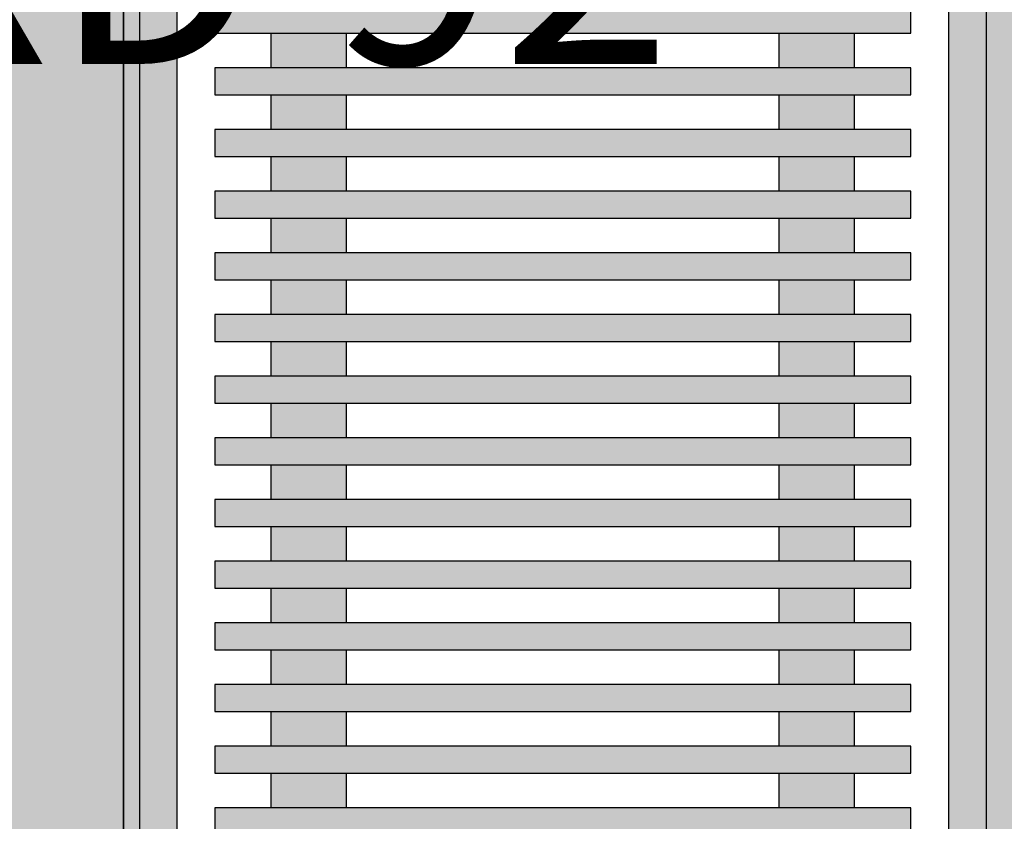
# Model space of a CAD drawing. Units: inches. Extents: x 1704 to 6393, y -157 to 1172.
# Tile 28 of 122: x 2351 to 2377, y 295 to 316. Entities that reach past the tile are written whole.
import ezdxf

# ---------------------------------------------------------------- set-up
doc = ezdxf.new("R2010")
doc.units = ezdxf.units.IN
doc.header["$MEASUREMENT"] = 0
for name, color, linetype, lineweight in [('A-ANNO-DIMS', 7, 'Continuous', 13), ('A-FURN', 8, 'Continuous', 18), ('A-WALL-PATT', 7, 'Continuous', 13), ('estofado', 7, 'Continuous', 25), ('WALLS', 7, 'Continuous', 35)]:
    doc.layers.add(name, color=color, linetype=linetype, lineweight=lineweight)
doc.layers.add('A-FLOR-PATT', color=7, linetype='Continuous', lineweight=13, true_color=0xf2f2f2)
doc.layers.add('MOBIL', color=7, linetype='Continuous')
doc.styles.get("Standard").update_dxf_attribs({"font": 'arial.ttf'})
doc.dimstyles.get("Standard").update_dxf_attribs({"dimtxt": 6, "dimasz": 2, "dimexe": 0.18, "dimexo": 0.0625, "dimgap": 0.09, "dimtad": 0, "dimtih": 1, "dimtoh": 1, "dimdec": 1, "dimzin": 0, "dimdsep": 46, "dimlunit": 3, "dimtxsty": 'Standard', "dimblk": 'ARCHTICK', "dimcen": 0.09, "dimadec": 0, "dimazin": 0, "dimtfac": 1, "dimtdec": 1, "dimtofl": 0, "dimtmove": 0, "dimatfit": 3, "dimfxl": 1, "dimtolj": 1, "dimtzin": 0, "dimarcsym": 0})

# ---------------------------------------------------------------- blocks, each defined once
blk = doc.blocks.new('Aparador Aido WV')
at = {"layer": 'MOBIL'}
h = blk.add_hatch(color=256, dxfattribs=at)
h.set_gradient(color1=(226, 228, 228), one_color=1, tint=1, name='CYLINDER')
h.paths.add_polyline_path([(0.9, -0.02), (0.9, 0), (-0.9, 0), (-0.9, -0.02)])
h = blk.add_hatch(color=256, dxfattribs=at)
h.set_gradient(color1=(106, 79, 62), color2=(55, 41, 32), one_color=1, tint=0.17)
h.paths.add_polyline_path([(-0.4692, -0.04017), (-0.4692, -0.40983), (-0.45483, -0.40983), (-0.45483, -0.04017)])
h = blk.add_hatch(color=256, dxfattribs=at)
h.set_gradient(color1=(106, 79, 62), color2=(55, 41, 32), one_color=1, tint=0.17)
h.paths.add_polyline_path([(-0.43644, -0.04017), (-0.43644, -0.40983), (-0.42208, -0.40983), (-0.42208, -0.04017)])
h = blk.add_hatch(color=256, dxfattribs=at)
h.set_gradient(color1=(106, 79, 62), color2=(55, 41, 32), one_color=1, tint=0.17)
h.paths.add_polyline_path([(-0.40369, -0.04017), (-0.40369, -0.40983), (-0.38933, -0.40983), (-0.38933, -0.04017)])
h = blk.add_hatch(color=256, dxfattribs=at)
h.set_gradient(color1=(106, 79, 62), color2=(55, 41, 32), one_color=1, tint=0.17)
h.paths.add_polyline_path([(-0.37094, -0.04017), (-0.37094, -0.40983), (-0.35658, -0.40983), (-0.35658, -0.04017)])
h = blk.add_hatch(color=256, dxfattribs=at)
h.set_gradient(color1=(106, 79, 62), color2=(55, 41, 32), one_color=1, tint=0.17)
h.paths.add_polyline_path([(-0.33819, -0.04017), (-0.33819, -0.40983), (-0.32382, -0.40983), (-0.32382, -0.04017)])
h = blk.add_hatch(color=256, dxfattribs=at)
h.set_gradient(color1=(106, 79, 62), color2=(55, 41, 32), one_color=1, tint=0.17)
h.paths.add_polyline_path([(-0.30544, -0.04017), (-0.30544, -0.40983), (-0.29107, -0.40983), (-0.29107, -0.04017)])
h = blk.add_hatch(color=256, dxfattribs=at)
h.set_gradient(color1=(106, 79, 62), color2=(55, 41, 32), one_color=1, tint=0.17)
h.paths.add_polyline_path([(-0.27269, -0.04017), (-0.27269, -0.40983), (-0.25832, -0.40983), (-0.25832, -0.04017)])
h = blk.add_hatch(color=256, dxfattribs=at)
h.set_gradient(color1=(106, 79, 62), color2=(55, 41, 32), one_color=1, tint=0.17)
h.paths.add_polyline_path([(-0.23993, -0.04017), (-0.23993, -0.40983), (-0.22557, -0.40983), (-0.22557, -0.04017)])
h = blk.add_hatch(color=256, dxfattribs=at)
h.set_gradient(color1=(106, 79, 62), color2=(55, 41, 32), one_color=1, tint=0.17)
h.paths.add_polyline_path([(-0.20718, -0.40983), (-0.19282, -0.40983), (-0.19282, -0.04017), (-0.20718, -0.04017)])
h = blk.add_hatch(color=256, dxfattribs=at)
h.set_gradient(color1=(106, 79, 62), color2=(55, 41, 32), one_color=1, tint=0.17)
h.paths.add_polyline_path([(-0.17443, -0.04017), (-0.17443, -0.40983), (-0.16007, -0.40983), (-0.16007, -0.04017)])
h = blk.add_hatch(color=256, dxfattribs=at)
h.set_gradient(color1=(106, 79, 62), color2=(55, 41, 32), one_color=1, tint=0.17)
h.paths.add_polyline_path([(-0.14168, -0.04017), (-0.14168, -0.40983), (-0.12731, -0.40983), (-0.12731, -0.04017)])
h = blk.add_hatch(color=256, dxfattribs=at)
h.set_gradient(color1=(106, 79, 62), color2=(55, 41, 32), one_color=1, tint=0.17)
h.paths.add_polyline_path([(-0.10893, -0.04017), (-0.10893, -0.40983), (-0.09456, -0.40983), (-0.09456, -0.04017)])
h = blk.add_hatch(color=256, dxfattribs=at)
h.set_gradient(color1=(106, 79, 62), color2=(55, 41, 32), one_color=1, tint=0.17)
h.paths.add_polyline_path([(-0.07618, -0.04017), (-0.07618, -0.40983), (-0.06181, -0.40983), (-0.06181, -0.04017)])
h = blk.add_hatch(color=256, dxfattribs=at)
h.set_gradient(color1=(106, 79, 62), color2=(55, 41, 32), one_color=1, tint=0.17)
h.paths.add_polyline_path([(-0.04342, -0.04017), (-0.04342, -0.40983), (-0.02906, -0.40983), (-0.02906, -0.04017)])
h = blk.add_hatch(color=256, dxfattribs=at)
h.set_gradient(color1=(106, 79, 62), color2=(157, 117, 92), one_color=1, tint=0.49)
h.paths.add_polyline_path([(-0.43644, -0.07), (-0.45483, -0.07), (-0.45483, -0.11), (-0.43644, -0.11)])
h = blk.add_hatch(color=256, dxfattribs=at)
h.set_gradient(color1=(106, 79, 62), color2=(157, 117, 92), one_color=1, tint=0.49)
h.paths.add_polyline_path([(-0.40369, -0.07), (-0.42208, -0.07), (-0.42208, -0.11), (-0.40369, -0.11)])
h = blk.add_hatch(color=256, dxfattribs=at)
h.set_gradient(color1=(106, 79, 62), color2=(157, 117, 92), one_color=1, tint=0.49)
h.paths.add_polyline_path([(-0.37094, -0.07), (-0.38933, -0.07), (-0.38933, -0.11), (-0.37094, -0.11)])
h = blk.add_hatch(color=256, dxfattribs=at)
h.set_gradient(color1=(106, 79, 62), color2=(157, 117, 92), one_color=1, tint=0.49)
h.paths.add_polyline_path([(-0.33819, -0.07), (-0.35658, -0.07), (-0.35658, -0.11), (-0.33819, -0.11)])
h = blk.add_hatch(color=256, dxfattribs=at)
h.set_gradient(color1=(106, 79, 62), color2=(157, 117, 92), one_color=1, tint=0.49)
h.paths.add_polyline_path([(-0.30544, -0.07), (-0.32382, -0.07), (-0.32382, -0.11), (-0.30544, -0.11)])
h = blk.add_hatch(color=256, dxfattribs=at)
h.set_gradient(color1=(106, 79, 62), color2=(157, 117, 92), one_color=1, tint=0.49)
h.paths.add_polyline_path([(-0.27269, -0.07), (-0.29107, -0.07), (-0.29107, -0.11), (-0.27269, -0.11)])
h = blk.add_hatch(color=256, dxfattribs=at)
h.set_gradient(color1=(106, 79, 62), color2=(157, 117, 92), one_color=1, tint=0.49)
h.paths.add_polyline_path([(-0.23993, -0.07), (-0.25832, -0.07), (-0.25832, -0.11), (-0.23993, -0.11)])
h = blk.add_hatch(color=256, dxfattribs=at)
h.set_gradient(color1=(106, 79, 62), color2=(157, 117, 92), one_color=1, tint=0.49)
h.paths.add_polyline_path([(-0.20718, -0.07), (-0.22557, -0.07), (-0.22557, -0.11), (-0.20718, -0.11)])
h = blk.add_hatch(color=256, dxfattribs=at)
h.set_gradient(color1=(106, 79, 62), color2=(157, 117, 92), one_color=1, tint=0.49)
h.paths.add_polyline_path([(-0.17443, -0.07), (-0.19282, -0.07), (-0.19282, -0.11), (-0.17443, -0.11)])
h = blk.add_hatch(color=256, dxfattribs=at)
h.set_gradient(color1=(106, 79, 62), color2=(157, 117, 92), one_color=1, tint=0.49)
h.paths.add_polyline_path([(-0.14168, -0.07), (-0.16007, -0.07), (-0.16007, -0.11), (-0.14168, -0.11)])
h = blk.add_hatch(color=256, dxfattribs=at)
h.set_gradient(color1=(106, 79, 62), color2=(157, 117, 92), one_color=1, tint=0.49)
h.paths.add_polyline_path([(-0.10893, -0.07), (-0.12731, -0.07), (-0.12731, -0.11), (-0.10893, -0.11)])
h = blk.add_hatch(color=256, dxfattribs=at)
h.set_gradient(color1=(106, 79, 62), color2=(157, 117, 92), one_color=1, tint=0.49)
h.paths.add_polyline_path([(-0.07618, -0.07), (-0.09456, -0.07), (-0.09456, -0.11), (-0.07618, -0.11)])
h = blk.add_hatch(color=256, dxfattribs=at)
h.set_gradient(color1=(106, 79, 62), color2=(157, 117, 92), one_color=1, tint=0.49)
h.paths.add_polyline_path([(-0.04342, -0.07), (-0.06181, -0.07), (-0.06181, -0.11), (-0.04342, -0.11)])
h = blk.add_hatch(color=256, dxfattribs=at)
h.set_gradient(color1=(106, 79, 62), color2=(157, 117, 92), one_color=1, tint=0.49)
h.paths.add_polyline_path([(-0.43644, -0.34), (-0.45483, -0.34), (-0.45483, -0.38), (-0.43644, -0.38)])
h = blk.add_hatch(color=256, dxfattribs=at)
h.set_gradient(color1=(106, 79, 62), color2=(157, 117, 92), one_color=1, tint=0.49)
h.paths.add_polyline_path([(-0.40369, -0.34), (-0.42208, -0.34), (-0.42208, -0.38), (-0.40369, -0.38)])
h = blk.add_hatch(color=256, dxfattribs=at)
h.set_gradient(color1=(106, 79, 62), color2=(157, 117, 92), one_color=1, tint=0.49)
h.paths.add_polyline_path([(-0.37094, -0.34), (-0.38933, -0.34), (-0.38933, -0.38), (-0.37094, -0.38)])
h = blk.add_hatch(color=256, dxfattribs=at)
h.set_gradient(color1=(106, 79, 62), color2=(157, 117, 92), one_color=1, tint=0.49)
h.paths.add_polyline_path([(-0.33819, -0.34), (-0.35658, -0.34), (-0.35658, -0.38), (-0.33819, -0.38)])
h = blk.add_hatch(color=256, dxfattribs=at)
h.set_gradient(color1=(106, 79, 62), color2=(157, 117, 92), one_color=1, tint=0.49)
h.paths.add_polyline_path([(-0.30544, -0.34), (-0.32382, -0.34), (-0.32382, -0.38), (-0.30544, -0.38)])
h = blk.add_hatch(color=256, dxfattribs=at)
h.set_gradient(color1=(106, 79, 62), color2=(157, 117, 92), one_color=1, tint=0.49)
h.paths.add_polyline_path([(-0.27269, -0.34), (-0.29107, -0.34), (-0.29107, -0.38), (-0.27269, -0.38)])
h = blk.add_hatch(color=256, dxfattribs=at)
h.set_gradient(color1=(106, 79, 62), color2=(157, 117, 92), one_color=1, tint=0.49)
h.paths.add_polyline_path([(-0.23993, -0.34), (-0.25832, -0.34), (-0.25832, -0.38), (-0.23993, -0.38)])
h = blk.add_hatch(color=256, dxfattribs=at)
h.set_gradient(color1=(106, 79, 62), color2=(157, 117, 92), one_color=1, tint=0.49)
h.paths.add_polyline_path([(-0.20718, -0.34), (-0.22557, -0.34), (-0.22557, -0.38), (-0.20718, -0.38)])
h = blk.add_hatch(color=256, dxfattribs=at)
h.set_gradient(color1=(106, 79, 62), color2=(157, 117, 92), one_color=1, tint=0.49)
h.paths.add_polyline_path([(-0.17443, -0.34), (-0.19282, -0.34), (-0.19282, -0.38), (-0.17443, -0.38)])
h = blk.add_hatch(color=256, dxfattribs=at)
h.set_gradient(color1=(106, 79, 62), color2=(157, 117, 92), one_color=1, tint=0.49)
h.paths.add_polyline_path([(-0.14168, -0.34), (-0.16007, -0.34), (-0.16007, -0.38), (-0.14168, -0.38)])
h = blk.add_hatch(color=256, dxfattribs=at)
h.set_gradient(color1=(106, 79, 62), color2=(157, 117, 92), one_color=1, tint=0.49)
h.paths.add_polyline_path([(-0.10893, -0.34), (-0.12731, -0.34), (-0.12731, -0.38), (-0.10893, -0.38)])
h = blk.add_hatch(color=256, dxfattribs=at)
h.set_gradient(color1=(106, 79, 62), color2=(157, 117, 92), one_color=1, tint=0.49)
h.paths.add_polyline_path([(-0.07618, -0.34), (-0.09456, -0.34), (-0.09456, -0.38), (-0.07618, -0.38)])
h = blk.add_hatch(color=256, dxfattribs=at)
h.set_gradient(color1=(106, 79, 62), color2=(157, 117, 92), one_color=1, tint=0.49)
h.paths.add_polyline_path([(-0.04342, -0.34), (-0.06181, -0.34), (-0.06181, -0.38), (-0.04342, -0.38)])
h = blk.add_hatch(color=256, dxfattribs=at)
h.set_gradient(color1=(226, 228, 228), one_color=1, tint=1, name='CYLINDER')
h.paths.add_polyline_path([(0.9, -0.45), (0.9, -0.43), (-0.9, -0.43), (-0.9, -0.45)])
at = {"layer": 'estofado', "ltscale": 0.5}
for p, q in [((-0.45483, -0.07), (-0.43644, -0.07)), ((-0.42208, -0.07), (-0.40369, -0.07)), ((-0.38933, -0.07), (-0.37094, -0.07)), ((-0.35658, -0.07), (-0.33819, -0.07)), ((-0.32382, -0.07), (-0.30544, -0.07)), ((-0.29107, -0.07), (-0.27269, -0.07)), ((-0.25832, -0.07), (-0.23993, -0.07)), ((-0.22557, -0.07), (-0.20718, -0.07)), ((-0.19282, -0.07), (-0.17443, -0.07)), ((-0.16007, -0.07), (-0.14168, -0.07)), ((-0.12731, -0.07), (-0.10893, -0.07)), ((-0.09456, -0.07), (-0.07618, -0.07)), ((-0.06181, -0.07), (-0.04342, -0.07)), ((-0.45483, -0.11), (-0.43644, -0.11)), ((-0.42208, -0.11), (-0.40369, -0.11)), ((-0.38933, -0.11), (-0.37094, -0.11)), ((-0.35658, -0.11), (-0.33819, -0.11)), ((-0.32382, -0.11), (-0.30544, -0.11)), ((-0.29107, -0.11), (-0.27269, -0.11)), ((-0.25832, -0.11), (-0.23993, -0.11)), ((-0.22557, -0.11), (-0.20718, -0.11)), ((-0.19282, -0.11), (-0.17443, -0.11)), ((-0.16007, -0.11), (-0.14168, -0.11)), ((-0.12731, -0.11), (-0.10893, -0.11)), ((-0.09456, -0.11), (-0.07618, -0.11)), ((-0.06181, -0.11), (-0.04342, -0.11)), ((-0.45483, -0.34), (-0.43644, -0.34)), ((-0.42208, -0.34), (-0.40369, -0.34)), ((-0.38933, -0.34), (-0.37094, -0.34)), ((-0.35658, -0.34), (-0.33819, -0.34)), ((-0.32382, -0.34), (-0.30544, -0.34)), ((-0.29107, -0.34), (-0.27269, -0.34)), ((-0.25832, -0.34), (-0.23993, -0.34)), ((-0.22557, -0.34), (-0.20718, -0.34)), ((-0.19282, -0.34), (-0.17443, -0.34)), ((-0.16007, -0.34), (-0.14168, -0.34)), ((-0.12731, -0.34), (-0.10893, -0.34)), ((-0.09456, -0.34), (-0.07618, -0.34)), ((-0.06181, -0.34), (-0.04342, -0.34)), ((-0.45483, -0.38), (-0.43644, -0.38)), ((-0.42208, -0.38), (-0.40369, -0.38)), ((-0.38933, -0.38), (-0.37094, -0.38)), ((-0.35658, -0.38), (-0.33819, -0.38)), ((-0.32382, -0.38), (-0.30544, -0.38)), ((-0.29107, -0.38), (-0.27269, -0.38)), ((-0.25832, -0.38), (-0.23993, -0.38)), ((-0.22557, -0.38), (-0.20718, -0.38)), ((-0.19282, -0.38), (-0.17443, -0.38)), ((-0.16007, -0.38), (-0.14168, -0.38)), ((-0.12731, -0.38), (-0.10893, -0.38)), ((-0.09456, -0.38), (-0.07618, -0.38)), ((-0.06181, -0.38), (-0.04342, -0.38))]:
    blk.add_line(p, q, dxfattribs=at)
for points in [[(-0.4692, -0.04017), (-0.4692, -0.40983), (-0.45483, -0.40983), (-0.45483, -0.04017)], [(-0.43644, -0.04017), (-0.43644, -0.40983), (-0.42208, -0.40983), (-0.42208, -0.04017)], [(-0.40369, -0.04017), (-0.40369, -0.40983), (-0.38933, -0.40983), (-0.38933, -0.04017)], [(-0.37094, -0.04017), (-0.37094, -0.40983), (-0.35658, -0.40983), (-0.35658, -0.04017)], [(-0.33819, -0.04017), (-0.33819, -0.40983), (-0.32382, -0.40983), (-0.32382, -0.04017)], [(-0.30544, -0.04017), (-0.30544, -0.40983), (-0.29107, -0.40983), (-0.29107, -0.04017)], [(-0.27269, -0.04017), (-0.27269, -0.40983), (-0.25832, -0.40983), (-0.25832, -0.04017)], [(-0.23993, -0.04017), (-0.23993, -0.40983), (-0.22557, -0.40983), (-0.22557, -0.04017)], [(-0.20718, -0.04017), (-0.20718, -0.40983), (-0.19282, -0.40983), (-0.19282, -0.04017)], [(-0.17443, -0.04017), (-0.17443, -0.40983), (-0.16007, -0.40983), (-0.16007, -0.04017)], [(-0.14168, -0.04017), (-0.14168, -0.40983), (-0.12731, -0.40983), (-0.12731, -0.04017)], [(-0.10893, -0.04017), (-0.10893, -0.40983), (-0.09456, -0.40983), (-0.09456, -0.04017)], [(-0.07618, -0.04017), (-0.07618, -0.40983), (-0.06181, -0.40983), (-0.06181, -0.04017)], [(-0.04342, -0.04017), (-0.04342, -0.40983), (-0.02906, -0.40983), (-0.02906, -0.04017)]]:
    blk.add_lwpolyline(points, close=True, dxfattribs=at)
at = {"layer": 'MOBIL'}
for p, q in [((0.9, -0.02), (-0.9, -0.02)), ((-0.9, -0.43), (0.9, -0.43))]:
    blk.add_line(p, q, dxfattribs=at)
blk.add_lwpolyline([(-0.9, -0.45), (0.9, -0.45), (0.9, 0), (-0.9, 0)], close=True, dxfattribs=at)
blk = doc.blocks.new('_ArchTick')
at = {"color": 0, "linetype": 'ByBlock', "const_width": 0.15}
blk.add_lwpolyline([(-0.5, -0.5), (0.5, 0.5)], dxfattribs=at)
blk = doc.blocks.new('*D68')
at = {"layer": 'A-ANNO-DIMS', "color": 0, "lineweight": -2, "transparency": 16777216}
for p, q in [((2353.706, 363.767), (2339.834, 363.767)), ((2340.014, 363.767), (2340.014, 321.111)), ((2340.014, 272.066), (2340.014, 314.722)), ((2353.706, 272.066), (2339.834, 272.066))]:
    blk.add_line(p, q, dxfattribs=at)
at = {"layer": 'Defpoints', "color": 0, "lineweight": -3, "transparency": 16777216}
for p in [(2340.014, 363.767), (2353.769, 363.767), (2353.769, 272.066)]:
    blk.add_point(p, dxfattribs=at)
at = {"layer": 'A-ANNO-DIMS', "color": 0, "lineweight": -2, "transparency": 16777216, "xscale": 2, "yscale": 2, "zscale": 2}
for p, rotation in [((2340.014, 363.767), 90), ((2340.014, 272.066), 270)]:
    blk.add_blockref('_ArchTick', p, dxfattribs=dict(at, rotation=rotation))
at = {"layer": 'A-ANNO-DIMS', "color": 0, "transparency": 16777216, "insert": (2340.014, 317.916), "char_height": 6, "attachment_point": 5}
blk.add_mtext('\\A1;SIDEBOARD 92', dxfattribs=at)
blk = doc.blocks.new('*D93')
at = {"layer": 'A-ANNO-DIMS', "color": 0, "lineweight": -2, "transparency": 16777216}
for p, q in [((2605.286, 895.213), (1829.698, 895.213)), ((1829.878, 895.213), (1829.878, 495.866)), ((1829.878, 90.213), (1829.878, 489.56)), ((2605.286, 90.213), (1829.698, 90.213))]:
    blk.add_line(p, q, dxfattribs=at)
at = {"layer": 'Defpoints', "color": 0, "lineweight": -3, "transparency": 16777216}
for p in [(2605.349, 895.213), (1829.878, 90.213), (2605.349, 90.213)]:
    blk.add_point(p, dxfattribs=at)
at = {"layer": 'A-ANNO-DIMS', "color": 0, "lineweight": -2, "transparency": 16777216, "xscale": 2, "yscale": 2, "zscale": 2}
for p, rotation in [((1829.878, 895.213), 90), ((1829.878, 90.213), 270)]:
    blk.add_blockref('_ArchTick', p, dxfattribs=dict(at, rotation=rotation))
at = {"layer": 'A-ANNO-DIMS', "color": 0, "transparency": 16777216, "insert": (1829.878, 492.713), "char_height": 6, "attachment_point": 5}
blk.add_mtext('\\A1;805', dxfattribs=at)

msp = doc.modelspace()

# ---------------------------------------------------------------- hatches: boundary and pattern name
at = {"layer": 'A-FLOR-PATT', "transparency": 33554528}
h = msp.add_hatch(color=256, dxfattribs=at)
h.dxf.hatch_style = 1
h.paths.add_polyline_path([(2325.349, 863.213), (2325.349, 887.213), (2263.349, 887.213), (2167.349, 887.213), (2081.349, 887.213), (2081.349, 719.213), (2277.349, 719.213), (2277.349, 711.213), (2277.349, 372.213), (2349.349, 372.213), (2381.349, 372.213), (2381.349, 364.213), (2353.349, 364.213), (2353.349, 270.213), (2381.349, 270.213), (2381.349, 266.213), (2357.349, 266.213), (2357.349, 98.213), (2381.349, 98.213), (2385.181, 98.213), (2386.482, 98.213), (2424.215, 98.213), (2425.516, 98.213), (2429.349, 98.213), (2597.349, 98.213), (2597.349, 146.213), (2597.349, 218.213), (2597.349, 266.213), (2423.349, 266.213), (2423.349, 270.213), (2473.349, 270.213), (2473.349, 294.213), (2477.349, 294.213), (2477.349, 270.213), (2547.349, 270.213), (2547.349, 364.213), (2477.349, 364.213), (2477.349, 318.213), (2473.349, 318.213), (2473.349, 364.213), (2423.349, 364.213), (2423.349, 372.213), (2469.349, 372.213), (2469.349, 459.213), (2469.349, 538.213), (2350.349, 538.213), (2350.349, 565.713), (2358.349, 565.713), (2358.349, 545.213), (2420.349, 545.213), (2420.349, 610.213), (2358.349, 610.213), (2358.349, 589.713), (2350.349, 589.713), (2350.349, 615.213), (2425.349, 615.213), (2425.349, 607.213), (2425.349, 546.213), (2469.349, 546.213), (2514.349, 546.213), (2514.349, 607.213), (2449.349, 607.213), (2449.349, 615.213), (2451.738, 615.213), (2451.738, 659.213), (2427.738, 659.213), (2427.738, 665.213), (2367.738, 665.213), (2367.738, 667.213), (2367.738, 711.213), (2325.349, 711.213), (2325.349, 719.213), (2325.349, 755.213), (2325.349, 763.213)])
h.paths.add_polyline_path([(2233.858, 822.533, -0.187247), (2233.858, 809.14), (2231.697, 808.804, 0.084893), (2233.131, 814.486), (2230.424, 814.486, -0.104258), (2228.553, 808.313), (2217.751, 807.156, -0.222222), (2217.751, 824.517), (2228.553, 823.359, -0.104258), (2230.424, 817.186), (2233.131, 817.186, 0.084893), (2231.697, 822.868)], flags=16)
h.paths.add_polyline_path([(2213.621, 833.197), (2213.621, 798.475), (2156.048, 798.475), (2156.048, 833.197)], flags=16)
h.paths.add_polyline_path([(2203.932, 848.099), (2205.089, 837.296, -0.222222), (2187.728, 837.296), (2188.885, 848.099, -0.104258), (2195.058, 849.969), (2195.058, 852.676, 0.084893), (2189.377, 851.242), (2189.712, 853.404, -0.187247), (2203.105, 853.404), (2203.44, 851.242, 0.084893), (2197.759, 852.676), (2197.759, 849.969, -0.104258)], flags=16)
h.paths.add_polyline_path([(2181.941, 837.296, -0.222222), (2164.58, 837.296), (2165.737, 848.099, -0.104258), (2171.91, 849.969), (2171.91, 852.676, 0.084893), (2166.229, 851.242), (2166.564, 853.404, -0.187247), (2179.957, 853.404), (2180.292, 851.242, 0.084893), (2174.611, 852.676), (2174.611, 849.969, -0.104258), (2180.784, 848.099)], flags=16)
h.paths.add_polyline_path([(2205.089, 794.376), (2203.932, 783.574, -0.104258), (2197.759, 781.703), (2197.759, 778.996, 0.084893), (2203.44, 780.43), (2203.105, 778.269, -0.187247), (2189.712, 778.269), (2189.377, 780.43, 0.084893), (2195.058, 778.996), (2195.058, 781.703, -0.104258), (2188.885, 783.574), (2187.728, 794.376, -0.222222)], flags=16)
h.paths.add_polyline_path([(2181.941, 794.376), (2180.784, 783.574, -0.104258), (2174.611, 781.703), (2174.611, 778.996, 0.084893), (2180.292, 780.43), (2179.957, 778.269, -0.187247), (2166.564, 778.269), (2166.229, 780.43, 0.084893), (2171.91, 778.996), (2171.91, 781.703, -0.104258), (2165.737, 783.574), (2164.58, 794.376, -0.222222)], flags=16)
h.paths.add_polyline_path([(2151.918, 807.156), (2141.116, 808.313, -0.104258), (2139.245, 814.486), (2136.539, 814.486, 0.084893), (2137.972, 808.804), (2135.811, 809.14, -0.187247), (2135.811, 822.533), (2137.972, 822.868, 0.084893), (2136.539, 817.186), (2139.245, 817.186, -0.104258), (2141.116, 823.359), (2151.918, 824.517, -0.222222)], flags=16)
h.paths.add_polyline_path([(2357.868, 363.41), (2358.814, 363.41, 0.75376)], flags=16)
h.paths.add_polyline_path([(2372.241, 363.117), (2372.248, 363.117), (2372.248, 363.343), (2371.302, 363.343), (2371.302, 363.139, -1.360391)], flags=16)
h.paths.add_polyline_path([(2371.309, 272.716), (2371.302, 272.716), (2371.302, 272.49), (2372.248, 272.49), (2372.248, 272.693, -1.360391)], flags=16)
h.paths.add_polyline_path([(2357.875, 272.716), (2357.868, 272.716), (2357.868, 272.49), (2358.814, 272.49), (2358.814, 272.693, -1.360391)], flags=16)
h.paths.add_polyline_path([(2353.769, 363.074), (2376.347, 363.074), (2376.347, 272.759), (2353.769, 272.759)], flags=16)
h.paths.add_polyline_path([(2354.772, 362.07), (2375.344, 362.07), (2375.344, 273.762), (2354.772, 273.762)], flags=0)
h.paths.add_polyline_path([(2357.868, 363.343), (2358.814, 363.343), (2358.814, 363.117), (2357.868, 363.117)], flags=16)
h.paths.add_polyline_path([(2359.288, 359.184), (2359.288, 360.063), (2370.828, 360.063), (2370.828, 359.184), (2374.332, 359.184), (2374.332, 358.464), (2372.835, 358.464), (2372.835, 357.541), (2374.332, 357.541), (2374.332, 356.82), (2372.835, 356.82), (2372.835, 355.898), (2374.332, 355.898), (2374.332, 355.177), (2372.835, 355.177), (2372.835, 354.254), (2374.332, 354.254), (2374.332, 353.534), (2372.835, 353.534), (2372.835, 352.611), (2374.332, 352.611), (2374.332, 351.89), (2372.835, 351.89), (2372.835, 350.968), (2374.332, 350.968), (2374.332, 350.247), (2372.835, 350.247), (2372.835, 349.324), (2374.332, 349.324), (2374.332, 348.604), (2372.835, 348.604), (2372.835, 347.681), (2374.332, 347.681), (2374.332, 346.96), (2372.835, 346.96), (2372.835, 346.038), (2374.332, 346.038), (2374.332, 345.317), (2372.835, 345.317), (2372.835, 344.395), (2374.332, 344.395), (2374.332, 343.674), (2372.835, 343.674), (2372.835, 342.751), (2374.332, 342.751), (2374.332, 342.03), (2372.835, 342.03), (2372.835, 341.108), (2374.332, 341.108), (2374.332, 340.387), (2372.835, 340.387), (2372.835, 339.465), (2374.332, 339.465), (2374.332, 338.744), (2372.835, 338.744), (2372.835, 337.821), (2374.332, 337.821), (2374.332, 337.1), (2372.835, 337.1), (2372.835, 336.178), (2374.332, 336.178), (2374.332, 335.457), (2372.835, 335.457), (2372.835, 334.535), (2374.332, 334.535), (2374.332, 333.814), (2372.835, 333.814), (2372.835, 332.891), (2374.332, 332.891), (2374.332, 332.171), (2372.835, 332.171), (2372.835, 331.248), (2374.332, 331.248), (2374.332, 330.527), (2372.835, 330.527), (2372.835, 329.605), (2374.332, 329.605), (2374.332, 328.884), (2372.835, 328.884), (2372.835, 327.961), (2374.332, 327.961), (2374.332, 327.241), (2372.835, 327.241), (2372.835, 326.318), (2374.332, 326.318), (2374.332, 325.597), (2372.835, 325.597), (2372.835, 324.675), (2374.332, 324.675), (2374.332, 323.954), (2372.835, 323.954), (2372.835, 323.031), (2374.332, 323.031), (2374.332, 322.311), (2372.835, 322.311), (2372.835, 321.388), (2374.332, 321.388), (2374.332, 320.667), (2372.835, 320.667), (2372.835, 319.745), (2374.332, 319.745), (2374.332, 319.024), (2372.835, 319.024), (2372.835, 318.102), (2374.332, 318.102), (2374.332, 317.381), (2372.835, 317.381), (2372.835, 316.458), (2374.332, 316.458), (2374.332, 315.737), (2372.835, 315.737), (2372.835, 314.815), (2374.332, 314.815), (2374.332, 314.094), (2372.835, 314.094), (2372.835, 313.172), (2374.332, 313.172), (2374.332, 312.451), (2372.835, 312.451), (2372.835, 311.528), (2374.332, 311.528), (2374.332, 310.807), (2372.835, 310.807), (2372.835, 309.885), (2374.332, 309.885), (2374.332, 309.164), (2372.835, 309.164), (2372.835, 308.242), (2374.332, 308.242), (2374.332, 307.521), (2372.835, 307.521), (2372.835, 306.598), (2374.332, 306.598), (2374.332, 305.878), (2372.835, 305.878), (2372.835, 304.955), (2374.332, 304.955), (2374.332, 304.234), (2372.835, 304.234), (2372.835, 303.312), (2374.332, 303.312), (2374.332, 302.591), (2372.835, 302.591), (2372.835, 301.668), (2374.332, 301.668), (2374.332, 300.948), (2372.835, 300.948), (2372.835, 300.025), (2374.332, 300.025), (2374.332, 299.304), (2372.835, 299.304), (2372.835, 298.382), (2374.332, 298.382), (2374.332, 297.661), (2372.835, 297.661), (2372.835, 296.738), (2374.332, 296.738), (2374.332, 296.018), (2372.835, 296.018), (2372.835, 295.095), (2374.332, 295.095), (2374.332, 294.374), (2372.835, 294.374), (2372.835, 293.452), (2374.332, 293.452), (2374.332, 292.731), (2372.835, 292.731), (2372.835, 291.809), (2374.332, 291.809), (2374.332, 291.088), (2372.835, 291.088), (2372.835, 290.165), (2374.332, 290.165), (2374.332, 289.444), (2372.835, 289.444), (2372.835, 288.522), (2374.332, 288.522), (2374.332, 287.801), (2372.835, 287.801), (2372.835, 286.879), (2374.332, 286.879), (2374.332, 286.158), (2372.835, 286.158), (2372.835, 285.235), (2374.332, 285.235), (2374.332, 284.514), (2372.835, 284.514), (2372.835, 283.592), (2374.332, 283.592), (2374.332, 282.871), (2372.835, 282.871), (2372.835, 281.949), (2374.332, 281.949), (2374.332, 281.228), (2372.835, 281.228), (2372.835, 280.305), (2374.332, 280.305), (2374.332, 279.585), (2372.835, 279.585), (2372.835, 278.662), (2374.332, 278.662), (2374.332, 277.941), (2372.835, 277.941), (2372.835, 277.019), (2374.332, 277.019), (2374.332, 276.298), (2370.828, 276.298), (2370.828, 275.769), (2359.288, 275.769), (2359.288, 276.298), (2355.784, 276.298), (2355.784, 277.019), (2357.281, 277.019), (2357.281, 277.941), (2355.784, 277.941), (2355.784, 278.662), (2357.281, 278.662), (2357.281, 279.585), (2355.784, 279.585), (2355.784, 280.305), (2357.281, 280.305), (2357.281, 281.228), (2355.784, 281.228), (2355.784, 281.949), (2357.281, 281.949), (2357.281, 282.871), (2355.784, 282.871), (2355.784, 283.592), (2357.281, 283.592), (2357.281, 284.514), (2355.784, 284.514), (2355.784, 285.235), (2357.281, 285.235), (2357.281, 286.158), (2355.784, 286.158), (2355.784, 286.879), (2357.281, 286.879), (2357.281, 287.801), (2355.784, 287.801), (2355.784, 288.522), (2357.281, 288.522), (2357.281, 289.444), (2355.784, 289.444), (2355.784, 290.165), (2357.281, 290.165), (2357.281, 291.088), (2355.784, 291.088), (2355.784, 291.809), (2357.281, 291.809), (2357.281, 292.731), (2355.784, 292.731), (2355.784, 293.452), (2357.281, 293.452), (2357.281, 294.374), (2355.784, 294.374), (2355.784, 295.095), (2357.281, 295.095), (2357.281, 296.018), (2355.784, 296.018), (2355.784, 296.738), (2357.281, 296.738), (2357.281, 297.661), (2355.784, 297.661), (2355.784, 298.382), (2357.281, 298.382), (2357.281, 299.304), (2355.784, 299.304), (2355.784, 300.025), (2357.281, 300.025), (2357.281, 300.948), (2355.784, 300.948), (2355.784, 301.668), (2357.281, 301.668), (2357.281, 302.591), (2355.784, 302.591), (2355.784, 303.312), (2357.281, 303.312), (2357.281, 304.234), (2355.784, 304.234), (2355.784, 304.955), (2357.281, 304.955), (2357.281, 305.878), (2355.784, 305.878), (2355.784, 306.598), (2357.281, 306.598), (2357.281, 307.521), (2355.784, 307.521), (2355.784, 308.242), (2357.281, 308.242), (2357.281, 309.164), (2355.784, 309.164), (2355.784, 309.885), (2357.281, 309.885), (2357.281, 310.807), (2355.784, 310.807), (2355.784, 311.528), (2357.281, 311.528), (2357.281, 312.451), (2355.784, 312.451), (2355.784, 313.172), (2357.281, 313.172), (2357.281, 314.094), (2355.784, 314.094), (2355.784, 314.815), (2357.281, 314.815), (2357.281, 315.737), (2355.784, 315.737), (2355.784, 316.458), (2357.281, 316.458), (2357.281, 317.381), (2355.784, 317.381), (2355.784, 318.102), (2357.281, 318.102), (2357.281, 319.024), (2355.784, 319.024), (2355.784, 319.745), (2357.281, 319.745), (2357.281, 320.667), (2355.784, 320.667), (2355.784, 321.388), (2357.281, 321.388), (2357.281, 322.311), (2355.784, 322.311), (2355.784, 323.031), (2357.281, 323.031), (2357.281, 323.954), (2355.784, 323.954), (2355.784, 324.675), (2357.281, 324.675), (2357.281, 325.597), (2355.784, 325.597), (2355.784, 326.318), (2357.281, 326.318), (2357.281, 327.241), (2355.784, 327.241), (2355.784, 327.961), (2357.281, 327.961), (2357.281, 328.884), (2355.784, 328.884), (2355.784, 329.605), (2357.281, 329.605), (2357.281, 330.527), (2355.784, 330.527), (2355.784, 331.248), (2357.281, 331.248), (2357.281, 332.171), (2355.784, 332.171), (2355.784, 332.891), (2357.281, 332.891), (2357.281, 333.814), (2355.784, 333.814), (2355.784, 334.535), (2357.281, 334.535), (2357.281, 335.457), (2355.784, 335.457), (2355.784, 336.178), (2357.281, 336.178), (2357.281, 337.1), (2355.784, 337.1), (2355.784, 337.821), (2357.281, 337.821), (2357.281, 338.744), (2355.784, 338.744), (2355.784, 339.465), (2357.281, 339.465), (2357.281, 340.387), (2355.784, 340.387), (2355.784, 341.108), (2357.281, 341.108), (2357.281, 342.03), (2355.784, 342.03), (2355.784, 342.751), (2357.281, 342.751), (2357.281, 343.674), (2355.784, 343.674), (2355.784, 344.395), (2357.281, 344.395), (2357.281, 345.317), (2355.784, 345.317), (2355.784, 346.038), (2357.281, 346.038), (2357.281, 346.96), (2355.784, 346.96), (2355.784, 347.681), (2357.281, 347.681), (2357.281, 348.604), (2355.784, 348.604), (2355.784, 349.324), (2357.281, 349.324), (2357.281, 350.247), (2355.784, 350.247), (2355.784, 350.968), (2357.281, 350.968), (2357.281, 351.89), (2355.784, 351.89), (2355.784, 352.611), (2357.281, 352.611), (2357.281, 353.534), (2355.784, 353.534), (2355.784, 354.254), (2357.281, 354.254), (2357.281, 355.177), (2355.784, 355.177), (2355.784, 355.898), (2357.281, 355.898), (2357.281, 356.82), (2355.784, 356.82), (2355.784, 357.541), (2357.281, 357.541), (2357.281, 358.464), (2355.784, 358.464), (2355.784, 359.184)], flags=0)
at = {"layer": 'A-WALL-PATT', "transparency": 33554643}
h = msp.add_hatch(color=256, dxfattribs=at)
h.dxf.hatch_style = 1
h.paths.add_polyline_path([(2167.349, 895.213), (2073.349, 895.213), (2073.349, 887.213), (2081.349, 887.213), (2167.349, 887.213)])
h.paths.add_polyline_path([(2465.349, 895.213), (2273.349, 895.213), (2273.349, 903.213), (2263.349, 903.213), (2263.349, 895.213), (2263.349, 887.213), (2325.349, 887.213), (2325.349, 863.213), (2333.349, 863.213), (2333.349, 887.213), (2465.349, 887.213)])
h.paths.add_polyline_path([(2533.349, 895.213), (2513.349, 895.213), (2513.349, 887.213), (2513.349, 861.213), (2517.349, 861.213), (2517.349, 887.213), (2533.349, 887.213)])
h.paths.add_polyline_path([(2605.349, 895.213), (2581.349, 895.213), (2581.349, 887.213), (2597.349, 887.213), (2597.349, 854.213), (2605.349, 854.213)])
h.paths.add_polyline_path([(2605.349, 752.213), (2629.349, 752.213), (2629.349, 716.213), (2605.349, 716.213), (2605.349, 712.213), (2719.349, 712.213), (2719.349, 716.213), (2631.349, 716.213), (2631.349, 754.213), (2605.349, 754.213), (2605.349, 794.213), (2597.349, 794.213), (2597.349, 787.213), (2517.349, 787.213), (2517.349, 813.213), (2513.349, 813.213), (2513.349, 783.213), (2517.349, 783.213), (2597.349, 783.213), (2597.349, 719.213), (2517.349, 719.213), (2517.349, 753.213), (2513.349, 753.213), (2513.349, 719.213), (2365.349, 719.213), (2365.349, 763.213), (2325.349, 763.213), (2325.349, 755.213), (2357.349, 755.213), (2357.349, 719.213), (2325.349, 719.213), (2325.349, 711.213), (2547.349, 711.213), (2547.349, 615.213), (2449.349, 615.213), (2449.349, 607.213), (2514.349, 607.213), (2514.349, 546.213), (2439.349, 546.213), (2425.349, 546.213), (2425.349, 607.213), (2425.349, 615.213), (2350.349, 615.213), (2350.349, 589.713), (2358.349, 589.713), (2358.349, 610.213), (2420.349, 610.213), (2420.349, 545.213), (2358.349, 545.213), (2358.349, 565.713), (2350.349, 565.713), (2350.349, 538.213), (2469.349, 538.213), (2469.349, 459.213), (2469.349, 372.213), (2423.349, 372.213), (2423.349, 364.213), (2473.349, 364.213), (2473.349, 318.213), (2477.349, 318.213), (2477.349, 364.213), (2547.349, 364.213), (2547.349, 352.213), (2549.349, 352.213), (2549.349, 364.213), (2597.349, 364.213), (2597.349, 328.213), (2549.349, 328.213), (2547.349, 328.213), (2547.349, 326.213), (2549.349, 326.213), (2597.349, 326.213), (2605.349, 326.213), (2605.349, 377.057), (2597.349, 377.057), (2597.349, 372.213), (2477.349, 372.213), (2477.349, 451.213), (2597.349, 451.213), (2605.349, 451.213), (2605.349, 459.213), (2597.349, 459.213), (2477.349, 459.213), (2477.349, 538.213), (2597.349, 538.213), (2597.349, 495.213), (2605.349, 495.213), (2605.349, 512.213), (2631.349, 512.213), (2631.349, 568.213), (2605.349, 568.213), (2605.349, 577.213), (2597.349, 577.213), (2597.349, 542.213), (2518.349, 542.213), (2518.349, 607.213), (2532.349, 607.213), (2605.349, 607.213), (2605.349, 615.213), (2597.349, 615.213), (2551.349, 615.213), (2551.349, 711.213), (2597.349, 711.213), (2597.349, 645.213), (2605.349, 645.213), (2605.349, 712.213), (2605.349, 716.213)])
h.paths.add_polyline_path([(2605.349, 566.213), (2629.349, 566.213), (2629.349, 514.213), (2605.349, 514.213)], flags=16)
h.paths.add_polyline_path([(2381.349, 372.213), (2349.349, 372.213), (2349.349, 202.213), (2337.349, 202.213), (2337.349, 194.213), (2349.349, 194.213), (2349.349, 90.213), (2349.349, 72.213), (2357.349, 72.213), (2357.349, 90.213), (2381.349, 90.213), (2381.349, 98.213), (2357.349, 98.213), (2357.349, 266.213), (2381.349, 266.213), (2381.349, 270.213), (2353.349, 270.213), (2353.349, 364.213), (2381.349, 364.213)])
h.paths.add_polyline_path([(2605.349, 302.213), (2597.349, 302.213), (2597.349, 270.213), (2477.349, 270.213), (2477.349, 294.213), (2473.349, 294.213), (2473.349, 270.213), (2423.349, 270.213), (2423.349, 266.213), (2597.349, 266.213), (2597.349, 218.213), (2605.349, 218.213)])
h.paths.add_polyline_path([(2605.349, 146.213), (2597.349, 146.213), (2597.349, 98.213), (2429.349, 98.213), (2429.349, 90.213), (2597.349, 90.213), (2597.349, 72.213), (2605.349, 72.213), (2605.349, 90.213)])
h.paths.add_polyline_path([(2225.349, 202.213), (2049.349, 202.213), (2049.349, 194.213), (2225.349, 194.213)])
h.paths.add_polyline_path([(2289.349, 202.213), (2277.349, 202.213), (2273.349, 202.213), (2269.516, 202.213), (2269.516, 194.213), (2273.349, 194.213), (2277.349, 194.213), (2289.349, 194.213)])
h.paths.add_polyline_path([(2273.349, 372.213), (2029.19, 372.213), (2029.19, 364.213), (2273.349, 364.213)])
h.paths.add_polyline_path([(2277.349, 545.213), (2213.349, 545.213), (2213.349, 573.213), (2205.349, 573.213), (2177.349, 573.213), (2177.349, 545.213), (2073.349, 545.213), (2073.349, 538.213), (2081.349, 538.213), (2277.349, 538.213)])
h.paths.add_polyline_path([(2181.349, 545.213), (2181.349, 569.213), (2205.349, 569.213), (2205.349, 545.213)], flags=16)
h.paths.add_polyline_path([(2277.349, 719.213), (2081.349, 719.213), (2073.349, 719.213), (2073.349, 711.213), (2154.575, 711.213), (2205.349, 711.213), (2205.349, 687.213), (2205.349, 629.213), (2213.349, 629.213), (2273.349, 629.213), (2273.349, 631.213), (2207.349, 631.213), (2207.349, 707.213), (2231.349, 707.213), (2231.349, 709.213), (2207.349, 709.213), (2207.349, 711.213), (2277.349, 711.213)])

# ---------------------------------------------------------------- linework, layer by layer
at = {"layer": 'WALLS'}
msp.add_line((2353.349, 270.213), (2353.349, 364.213), dxfattribs=at)

# ---------------------------------------------------------------- block references
at = {"layer": 'A-FURN', "xscale": 50.174952135231, "yscale": 50.174952135231, "zscale": 50.174952135231, "rotation": 90}
msp.add_blockref('Aparador Aido WV', (2353.769, 317.916), dxfattribs=at)

# ---------------------------------------------------------------- dimensions: what is measured, and where the dimension line sits
at = {"layer": 'A-ANNO-DIMS'}
dim = msp.add_linear_dim(base=(1829.878, 90.213), p1=(2605.349, 895.213), p2=(2605.349, 90.213), angle=90, dimstyle='Standard', override={"dimdec": 0, "dimlfac": 1, "dimrnd": 0, "dimzin": 0, "dimdsep": 46, "dimlunit": 2}, dxfattribs=at)
dim.commit()
dim.dimension.update_dxf_attribs({"geometry": '*D93', "text_midpoint": (1829.878, 492.713)})
dim = msp.add_linear_dim(base=(2340.014, 363.767), p1=(2353.769, 272.066), p2=(2353.769, 363.767), angle=90, text='SIDEBOARD <>', dimstyle='Standard', override={"dimdec": 0, "dimlfac": 1, "dimrnd": 0, "dimzin": 0, "dimdsep": 46, "dimlunit": 2}, dxfattribs=at)
dim.commit()
dim.dimension.update_dxf_attribs({"geometry": '*D68', "text_midpoint": (2340.014, 317.916)})

doc.saveas('drawing.dxf')
